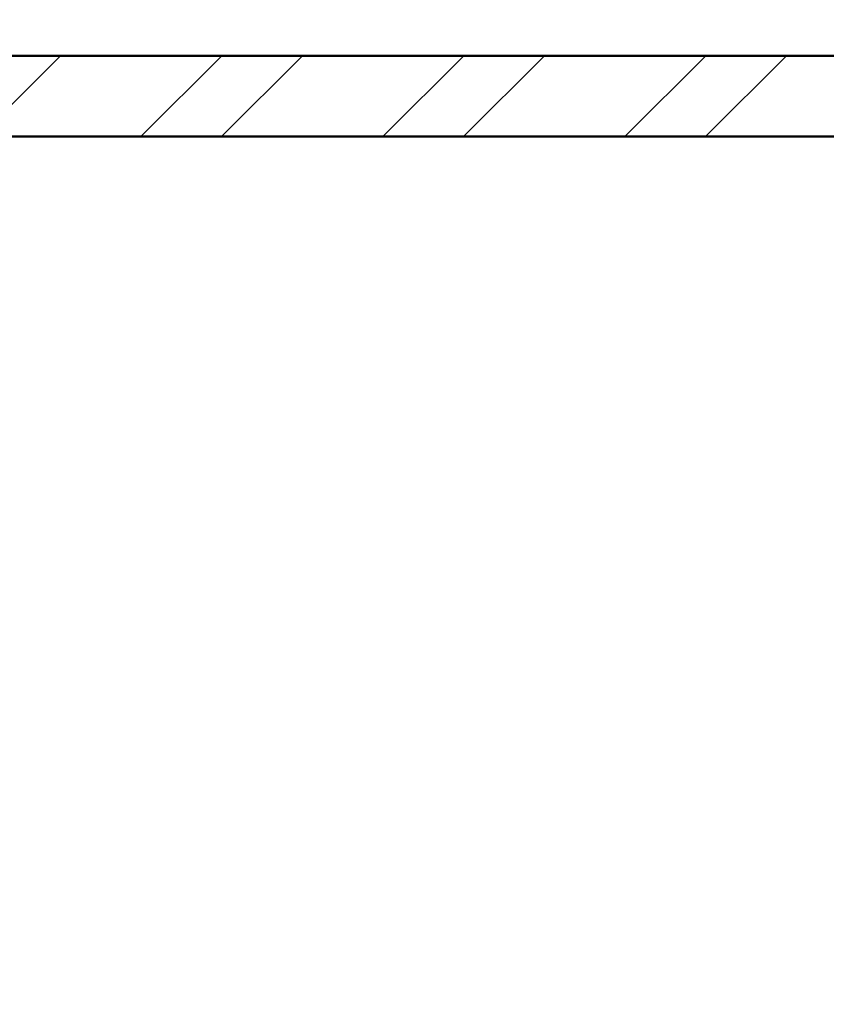
# Model space of a CAD drawing. Units: inches. Extents: x 1901 to 2863, y 888 to 2433.
# Tile 12 of 91: x 2199 to 2244, y 1403 to 1458. Entities that reach past the tile are written whole.
import ezdxf

# ---------------------------------------------------------------- set-up
doc = ezdxf.new("R2010")
doc.units = ezdxf.units.IN
doc.layers.add('A-WALL', color=7, linetype='Continuous', lineweight=50)
doc.layers.add('A-WALL-PATT', color=8, linetype='Continuous', lineweight=13)

msp = doc.modelspace()

# ---------------------------------------------------------------- hatches: boundary and pattern name
at = {"layer": 'A-WALL-PATT'}
h = msp.add_hatch(dxfattribs=at)
h.set_pattern_fill('ANSI32', color=256)
h.paths.add_polyline_path([(2192.501, 2274.134), (2141.264, 2274.134), (2141.264, 2269.634), (2192.501, 2269.634)])
h.paths.add_polyline_path([(2259.926, 2274.134), (2216.501, 2274.134), (2216.501, 2269.634), (2255.426, 2269.634), (2255.426, 2214.634), (2250.809, 2214.634), (2250.809, 2210.134), (2259.926, 2210.134), (2259.926, 2215.134), (2271.756, 2215.134), (2271.756, 2217.384), (2271.756, 2219.634), (2259.926, 2219.634)])
h.paths.add_polyline_path([(2171.426, 2269.634), (2166.926, 2269.634), (2166.926, 2219.634), (2121.238, 2219.634), (2121.238, 2215.134), (2166.926, 2215.134), (2166.926, 2083.134), (2161.807, 2083.134), (2161.807, 2078.634), (2171.426, 2078.634), (2176.996, 2078.634), (2176.996, 2080.884), (2176.996, 2083.134), (2171.426, 2083.134), (2171.426, 2210.134), (2230.912, 2210.134), (2230.912, 2212.384), (2230.912, 2214.634), (2171.426, 2214.634)])
h.paths.add_polyline_path([(2117.264, 2274.134), (2089.426, 2274.134), (2089.426, 2219.634), (2081.136, 2219.634), (2081.136, 2215.134), (2089.426, 2215.134), (2098.004, 2215.134), (2098.004, 2217.384), (2098.004, 2219.634), (2093.926, 2219.634), (2093.926, 2269.634), (2117.264, 2269.634), (2117.264, 2271.884)])
h.paths.add_polyline_path([(2343.426, 2219.634), (2329.295, 2219.634), (2329.295, 2215.134), (2338.926, 2215.134), (2338.926, 2184.739), (2343.426, 2184.739)])
h.paths.add_polyline_path([(2338.926, 2083.134), (2329.295, 2083.134), (2208.966, 2083.134), (2208.966, 2078.634), (2338.926, 2078.634)])
h.paths.add_polyline_path([(2343.426, 2136.739), (2338.926, 2136.739), (2338.926, 1872.634), (2343.426, 1872.634)])
h.paths.add_polyline_path([(2343.426, 1863.634), (2397.68, 1863.634), (2397.68, 1821.634), (2384.138, 1821.634), (2384.138, 1812.634), (2418.33, 1812.634), (2418.33, 1817.134), (2418.33, 1821.634), (2406.68, 1821.634), (2406.68, 1863.634), (2459.499, 1863.634), (2459.499, 1821.634), (2447.138, 1821.634), (2447.138, 1812.634), (2459.499, 1812.634), (2468.499, 1812.634), (2468.499, 1872.634), (2394.426, 1872.634), (2334.426, 1872.634), (2334.426, 1812.634), (2343.426, 1812.634), (2353.251, 1812.634), (2353.251, 1821.634), (2343.426, 1821.634)])
h.paths.add_polyline_path([(2510.014, 1872.634), (2468.499, 1872.634), (2468.499, 1868.134), (2510.014, 1868.134)])
h.paths.add_polyline_path([(2514.009, 1817.134), (2468.499, 1817.134), (2468.499, 1812.634), (2482.114, 1812.634), (2482.114, 1800.606), (2486.614, 1800.606), (2486.614, 1812.634), (2514.009, 1812.634)])
h.paths.add_polyline_path([(2299.247, 1814.884), (2299.247, 1817.134), (2295.926, 1817.134), (2295.926, 1854.169), (2293.676, 1854.169), (2291.426, 1854.169), (2291.426, 1817.134), (2266.109, 1817.134), (2266.109, 1812.634), (2299.247, 1812.634)])
h.paths.add_polyline_path([(2218.109, 1817.134), (2206.46, 1817.134), (2171.426, 1817.134), (2171.426, 1949.134), (2190.1, 1949.134), (2190.1, 1953.634), (2163.468, 1953.634), (2163.468, 1949.134), (2166.926, 1949.134), (2166.926, 1817.134), (2114.297, 1817.134), (2114.297, 1812.634), (2218.109, 1812.634)])
h.paths.add_polyline_path([(2029.426, 1970.922), (2024.926, 1970.922), (2024.926, 1912.717), (2029.426, 1912.717)])
h.paths.add_polyline_path([(2132.297, 1953.634), (2113.926, 1953.634), (2113.926, 1975.888), (2111.676, 1975.888), (2109.426, 1975.888), (2109.426, 1953.634), (2029.426, 1953.634), (2029.426, 1949.134), (2132.297, 1949.134)])
h.paths.add_polyline_path([(2029.426, 1853.606), (2029.31, 1853.606), (2029.31, 1853.606), (2029.426, 1853.606), (2029.426, 1864.717), (2024.926, 1864.717), (2024.926, 1812.634), (2066.297, 1812.634), (2066.297, 1814.884), (2066.297, 1817.134), (2029.426, 1817.134)])
h.paths.add_polyline_path([(2122.926, 2010.088), (2120.676, 2010.088), (2118.426, 2010.088), (2118.426, 2006.134), (2029.426, 2006.134), (2029.426, 2001.634), (2109.426, 2001.634), (2109.426, 1998.041), (2113.926, 1998.041), (2113.926, 2001.634), (2122.926, 2001.634)])
h.paths.add_polyline_path([(2029.426, 2031.376), (2024.926, 2031.376), (2024.926, 1994.922), (2027.176, 1994.922), (2029.426, 1994.922)])
h.paths.add_polyline_path([(2029.426, 2136.739), (2024.926, 2136.739), (2024.926, 2067.376), (2027.176, 2067.376), (2029.426, 2067.376)])
h.paths.add_polyline_path([(2125.618, 2083.134), (2029.426, 2083.134), (2029.426, 2078.634), (2118.426, 2078.634), (2118.426, 2030.715), (2122.926, 2030.715), (2122.926, 2078.634), (2125.618, 2078.634)])
h.paths.add_polyline_path([(2029.426, 2215.134), (2040.468, 2215.134), (2040.468, 2217.384), (2040.468, 2219.634), (2024.926, 2219.634), (2024.926, 2184.739), (2029.426, 2184.739), (2029.426, 2187.778)])
h.paths.add_polyline_path([(2686.426, 2274.134), (2659.284, 2274.134), (2659.284, 2269.634), (2681.926, 2269.634), (2681.926, 2219.634), (2676.816, 2219.634), (2676.816, 2215.134), (2681.926, 2215.134), (2697.011, 2215.134), (2697.011, 2217.384), (2697.011, 2219.634), (2686.426, 2219.634)])
h.paths.add_polyline_path([(2609.926, 2269.634), (2635.284, 2269.634), (2635.284, 2274.134), (2571.431, 2274.134), (2571.431, 2269.634), (2605.426, 2269.634), (2605.426, 2214.634), (2549.098, 2214.634), (2549.098, 2210.134), (2605.426, 2210.134), (2605.426, 2083.134), (2601.014, 2083.134), (2601.014, 2080.884), (2601.014, 2078.634), (2609.926, 2078.634), (2616.162, 2078.634), (2616.162, 2080.884), (2616.162, 2083.134), (2609.926, 2083.134), (2609.926, 2215.134), (2651.465, 2215.134), (2651.465, 2217.384), (2651.465, 2219.634), (2609.926, 2219.634)])
h.paths.add_polyline_path([(2521.426, 2269.634), (2547.431, 2269.634), (2547.431, 2271.884), (2547.431, 2274.134), (2516.926, 2274.134), (2516.926, 2219.634), (2506.41, 2219.634), (2506.41, 2215.134), (2516.926, 2215.134), (2516.926, 2210.134), (2525.402, 2210.134), (2525.402, 2212.384), (2525.402, 2214.634), (2521.426, 2214.634)])
h.paths.add_polyline_path([(2456.011, 2219.634), (2439.426, 2219.634), (2439.426, 2187.888), (2443.926, 2187.888), (2443.926, 2215.134), (2456.011, 2215.134)])
h.paths.add_polyline_path([(2752.926, 2219.634), (2739.485, 2219.634), (2739.485, 2215.134), (2748.426, 2215.134), (2748.426, 2187.888), (2752.926, 2187.888)])
h.paths.add_polyline_path([(2752.926, 2139.888), (2748.426, 2139.888), (2748.426, 2083.134), (2648.416, 2083.134), (2648.416, 2078.634), (2654.926, 2078.634), (2654.926, 2039.437), (2659.426, 2039.437), (2659.426, 2078.634), (2748.426, 2078.634), (2748.426, 2063.429), (2752.926, 2063.429)])
h.paths.add_polyline_path([(2752.926, 2010.634), (2659.426, 2010.634), (2659.426, 2015.652), (2654.926, 2015.652), (2654.926, 2010.634), (2605.426, 2010.634), (2605.426, 1920.967), (2609.926, 1920.967), (2609.926, 2006.134), (2748.426, 2006.134), (2748.426, 1982.466), (2752.926, 1982.466)])
h.paths.add_polyline_path([(2752.926, 2027.429), (2748.426, 2027.429), (2748.426, 2010.634), (2752.926, 2010.634)])
h.paths.add_polyline_path([(2748.426, 1886.134), (2609.926, 1886.134), (2609.926, 1889.719), (2605.426, 1889.719), (2605.426, 1861.262), (2609.926, 1861.262), (2609.926, 1881.634), (2748.426, 1881.634)])
h.paths.add_polyline_path([(2456.855, 2228.831), (2498.401, 2228.831), (2498.401, 2247.488), (2456.855, 2247.488)], flags=9)
h.paths.add_polyline_path([(2038.602, 2237.418), (2080.174, 2237.418), (2080.174, 2256.075), (2038.602, 2256.075)], flags=9)
h.paths.add_polyline_path([(2292.009, 1062.394), (2539.932, 1062.394), (2539.932, 1099.487), (2292.009, 1099.487)], flags=9)
h.paths.add_polyline_path([(2424.91, 1832.253), (2448.513, 1832.253), (2448.513, 1846.678), (2424.91, 1846.678)], flags=25)
h.paths.add_polyline_path([(2359.076, 1832.253), (2382.678, 1832.253), (2382.678, 1846.678), (2359.076, 1846.678)], flags=25)
h.paths.add_polyline_path([(2352.899, 1684.802), (2367.543, 1684.802), (2367.543, 1697.167), (2352.899, 1697.167)], flags=9)
h.paths.add_polyline_path([(2079.288, 1755.826), (2169.024, 1755.826), (2169.024, 1774.372), (2079.288, 1774.372)], flags=9)
h.paths.add_polyline_path([(2404.09, 1373.857), (2404.09, 1463.593), (2385.544, 1463.593), (2385.544, 1373.857)], flags=9)
h.paths.add_polyline_path([(2268.091, 2236.371), (2309.636, 2236.371), (2309.636, 2255.028), (2268.091, 2255.028)], flags=9)
h.paths.add_polyline_path([(2575.96, 1700.951), (2665.696, 1700.951), (2665.696, 1719.498), (2575.96, 1719.498)], flags=9)
h.paths.add_polyline_path([(2302.962, 1878.474), (2329.524, 1878.474), (2329.524, 1888.777), (2302.962, 1888.777)], flags=9)
h.paths.add_polyline_path([(2097.415, 2240.576), (2126.573, 2240.576), (2126.573, 2259.233), (2097.415, 2259.233)], flags=9)
h.paths.add_polyline_path([(2208.725, 2246.124), (2237.882, 2246.124), (2237.882, 2264.781), (2208.725, 2264.781)], flags=9)
h.paths.add_polyline_path([(2038.147, 1925.958), (2076.987, 1925.958), (2076.987, 1944.615), (2038.147, 1944.615)], flags=9)
h.paths.add_polyline_path([(2239.144, 1926.672), (2288.465, 1926.672), (2288.465, 1945.329), (2239.144, 1945.329)], flags=9)
h.paths.add_polyline_path([(2175.429, 2007.33), (2212.356, 2007.33), (2212.356, 2025.987), (2175.429, 2025.987)], flags=9)
h.paths.add_polyline_path([(2225.034, 2091.794), (2263.875, 2091.794), (2263.875, 2110.451), (2225.034, 2110.451)], flags=9)
h.paths.add_polyline_path([(2035.398, 2098.478), (2074.238, 2098.478), (2074.238, 2117.135), (2035.398, 2117.135)], flags=9)
h.paths.add_polyline_path([(2050.102, 2029.209), (2083.26, 2029.209), (2083.26, 2047.866), (2050.102, 2047.866)], flags=9)
h.paths.add_polyline_path([(2069.677, 1956.719), (2098.835, 1956.719), (2098.835, 1975.376), (2069.677, 1975.376)], flags=25)
h.paths.add_polyline_path([(2328.62, 1753.336), (2361.663, 1753.336), (2361.663, 1771.993), (2328.62, 1771.993)], flags=9)
h.paths.add_polyline_path([(2395.162, 2060.888), (2395.162, 2140.654), (2378.676, 2140.654), (2378.676, 2060.888)], flags=9)
h.paths.add_polyline_path([(2463.728, 2059.02), (2492.886, 2059.02), (2492.886, 2077.677), (2463.728, 2077.677)], flags=9)
h.paths.add_polyline_path([(2458.027, 2181.536), (2496.868, 2181.536), (2496.868, 2200.194), (2458.027, 2200.194)], flags=9)
h.paths.add_polyline_path([(2527.577, 2243.074), (2556.735, 2243.074), (2556.735, 2261.731), (2527.577, 2261.731)], flags=9)
h.paths.add_polyline_path([(2694.461, 2232.767), (2736.033, 2232.767), (2736.033, 2251.425), (2694.461, 2251.425)], flags=9)
h.paths.add_polyline_path([(2637.821, 2249.225), (2666.979, 2249.225), (2666.979, 2267.882), (2637.821, 2267.882)], flags=9)
h.paths.add_polyline_path([(2623.687, 2183.541), (2662.528, 2183.541), (2662.528, 2202.199), (2623.687, 2202.199)], flags=9)
h.paths.add_polyline_path([(2691.965, 2021.5), (2725.124, 2021.5), (2725.124, 2040.157), (2691.965, 2040.157)], flags=9)
h.paths.add_polyline_path([(2621.043, 1975.912), (2662.335, 1975.912), (2662.335, 1994.569), (2621.043, 1994.569)], flags=25)
h.paths.add_polyline_path([(2479.032, 1927.62), (2519.844, 1927.62), (2519.844, 1946.277), (2479.032, 1946.277)], flags=9)
h.paths.add_polyline_path([(2670.941, 1849.076), (2716.005, 1849.076), (2716.005, 1867.734), (2670.941, 1867.734)], flags=9)
h.paths.add_polyline_path([(2523.613, 1782.956), (2550.175, 1782.956), (2550.175, 1793.26), (2523.613, 1793.26)], flags=9)
h.paths.add_polyline_path([(2450.841, 1207.331), (2492.386, 1207.331), (2492.386, 1225.989), (2450.841, 1225.989)], flags=9)
h.paths.add_polyline_path([(2527.751, 1203.841), (2556.908, 1203.841), (2556.908, 1222.499), (2527.751, 1222.499)], flags=9)
h.paths.add_polyline_path([(2639.111, 1207.2), (2668.268, 1207.2), (2668.268, 1225.857), (2639.111, 1225.857)], flags=9)
h.paths.add_polyline_path([(2692.594, 1218.965), (2734.167, 1218.965), (2734.167, 1237.623), (2692.594, 1237.623)], flags=9)
h.paths.add_polyline_path([(2669.266, 1366.329), (2708.106, 1366.329), (2708.106, 1384.987), (2669.266, 1384.987)], flags=9)
h.paths.add_polyline_path([(2463.313, 1358.031), (2502.153, 1358.031), (2502.153, 1376.688), (2463.313, 1376.688)], flags=9)
h.paths.add_polyline_path([(2494.725, 1449.963), (2531.652, 1449.963), (2531.652, 1468.62), (2494.725, 1468.62)], flags=9)
h.paths.add_polyline_path([(2675.565, 1422.157), (2708.724, 1422.157), (2708.724, 1440.815), (2675.565, 1440.815)], flags=9)
h.paths.add_polyline_path([(2685.634, 1493.891), (2714.792, 1493.891), (2714.792, 1512.548), (2685.634, 1512.548)], flags=9)
h.paths.add_polyline_path([(2686.805, 1529.913), (2725.645, 1529.913), (2725.645, 1548.57), (2686.805, 1548.57)], flags=9)
h.paths.add_polyline_path([(2503.651, 1537.991), (2552.972, 1537.991), (2552.972, 1556.648), (2503.651, 1556.648)], flags=9)
h.paths.add_polyline_path([(2291.713, 1643.504), (2318.275, 1643.504), (2318.275, 1653.807), (2291.713, 1653.807)], flags=9)
h.paths.add_polyline_path([(2450.626, 1610.52), (2477.189, 1610.52), (2477.189, 1620.824), (2450.626, 1620.824)], flags=9)
h.paths.add_polyline_path([(2359.985, 1551.814), (2422.253, 1551.814), (2422.253, 1562.117), (2359.985, 1562.117)], flags=9)
h.paths.add_polyline_path([(2280.106, 1249.006), (2321.651, 1249.006), (2321.651, 1267.663), (2280.106, 1267.663)], flags=9)
h.paths.add_polyline_path([(2164.057, 1274.232), (2193.215, 1274.232), (2193.215, 1292.889), (2164.057, 1292.889)], flags=9)
h.paths.add_polyline_path([(2118.21, 1277.694), (2151.252, 1277.694), (2151.252, 1296.351), (2118.21, 1296.351)], flags=9)
h.paths.add_polyline_path([(2031.946, 1268.529), (2073.519, 1268.529), (2073.519, 1287.187), (2031.946, 1287.187)], flags=9)
h.paths.add_polyline_path([(2050.199, 1409.079), (2089.04, 1409.079), (2089.04, 1427.736), (2050.199, 1427.736)], flags=9)
h.paths.add_polyline_path([(2243.743, 1421.032), (2282.584, 1421.032), (2282.584, 1439.689), (2243.743, 1439.689)], flags=9)
h.paths.add_polyline_path([(2190.746, 1509.769), (2231.558, 1509.769), (2231.558, 1528.426), (2190.746, 1528.426)], flags=9)
h.paths.add_polyline_path([(2058.392, 1475.415), (2091.55, 1475.415), (2091.55, 1494.073), (2058.392, 1494.073)], flags=9)
h.paths.add_polyline_path([(2062.447, 1553.09), (2091.605, 1553.09), (2091.605, 1571.747), (2062.447, 1571.747)], flags=9)
h.paths.add_polyline_path([(2219.524, 1590.365), (2266.147, 1590.365), (2266.147, 1609.022), (2219.524, 1609.022)], flags=9)
h.paths.add_polyline_path([(2041.072, 1584.188), (2079.912, 1584.188), (2079.912, 1602.845), (2041.072, 1602.845)], flags=9)
h = msp.add_hatch(dxfattribs=at)
h.set_pattern_fill('ANSI32', color=256)
h.paths.add_polyline_path([(2443.926, 2139.888), (2439.426, 2139.888), (2439.426, 2069.348), (2441.676, 2069.348), (2443.926, 2069.348), (2443.926, 2078.634), (2521.926, 2078.634), (2521.926, 2075.067), (2524.176, 2075.067), (2526.426, 2075.067), (2526.426, 2078.634), (2571.755, 2078.634), (2571.755, 2080.884), (2571.755, 2083.134), (2443.926, 2083.134)])
h.paths.add_polyline_path([(2526.426, 2054.634), (2524.176, 2054.634), (2521.926, 2054.634), (2521.926, 2030.634), (2443.926, 2030.634), (2443.926, 2045.348), (2439.426, 2045.348), (2439.426, 1983.867), (2443.926, 1983.867), (2443.926, 2026.134), (2521.926, 2026.134), (2526.426, 2026.134)])
h.paths.add_polyline_path([(2443.926, 1923.867), (2439.426, 1923.867), (2439.426, 1872.634), (2443.926, 1872.634)])
h.paths.add_polyline_path([(2636.233, 1766.134), (2609.926, 1766.134), (2609.926, 1779.785), (2605.426, 1779.785), (2605.426, 1766.134), (2486.614, 1766.134), (2486.614, 1770.671), (2482.114, 1770.671), (2482.114, 1766.134), (2482.114, 1761.634), (2636.233, 1761.634), (2636.233, 1763.884)])
h.paths.add_polyline_path([(2519.536, 1663.384), (2519.536, 1665.634), (2494.926, 1665.634), (2481.831, 1665.634), (2481.831, 1663.384), (2481.831, 1661.134), (2490.426, 1661.134), (2490.426, 1640.157), (2494.926, 1640.157), (2494.926, 1661.134), (2519.536, 1661.134)])
h.paths.add_polyline_path([(2443.926, 1712.134), (2443.926, 1716.634), (2414.464, 1716.634), (2414.464, 1712.134), (2439.426, 1712.134), (2439.426, 1545.507), (2443.926, 1545.507), (2443.926, 1661.134), (2448.475, 1661.134), (2448.475, 1665.634), (2443.926, 1665.634)])
h.paths.add_polyline_path([(2343.426, 1712.134), (2365.525, 1712.134), (2365.525, 1714.384), (2365.525, 1716.634), (2333.871, 1716.634), (2333.871, 1714.384), (2333.871, 1712.134), (2338.926, 1712.134), (2338.926, 1575.634), (2338.926, 1545.507), (2343.426, 1545.507), (2343.426, 1547.507), (2343.426, 1580.134)])
h.paths.add_polyline_path([(2752.926, 1665.634), (2579.536, 1665.634), (2579.536, 1661.134), (2615.926, 1661.134), (2615.926, 1529.134), (2598.931, 1529.134), (2598.931, 1524.634), (2623.127, 1524.634), (2623.127, 1526.884), (2623.127, 1529.134), (2620.426, 1529.134), (2620.426, 1661.134), (2748.426, 1661.134), (2748.426, 1633.499), (2752.926, 1633.499)])
h.paths.add_polyline_path([(2752.926, 1419.929), (2748.426, 1419.929), (2748.426, 1400.134), (2659.426, 1400.134), (2659.426, 1444.333), (2657.176, 1444.333), (2654.926, 1444.333), (2654.926, 1400.134), (2643.649, 1400.134), (2643.649, 1395.634), (2748.426, 1395.634), (2748.426, 1364.035), (2752.926, 1364.035)])
h.paths.add_polyline_path([(2752.926, 1492.878), (2748.426, 1492.878), (2748.426, 1476.634), (2667.426, 1476.634), (2667.426, 1479.71), (2665.176, 1479.71), (2662.926, 1479.71), (2662.926, 1476.634), (2654.926, 1476.634), (2654.926, 1469.536), (2659.426, 1469.536), (2659.426, 1472.134), (2748.426, 1472.134), (2748.426, 1455.929), (2752.926, 1455.929)])
h.paths.add_polyline_path([(2752.926, 1304.035), (2748.426, 1304.035), (2748.426, 1263.634), (2738.66, 1263.634), (2738.66, 1259.134), (2752.926, 1259.134)])
h.paths.add_polyline_path([(2685.926, 1259.134), (2695.49, 1259.134), (2695.49, 1261.384), (2695.49, 1263.634), (2677.837, 1263.634), (2677.837, 1261.384), (2677.837, 1259.134), (2681.426, 1259.134), (2681.426, 1203.634), (2653.277, 1203.634), (2653.277, 1199.134), (2685.926, 1199.134), (2685.926, 1203.634)])
h.paths.add_polyline_path([(2609.426, 1395.634), (2611.848, 1395.634), (2611.848, 1400.134), (2598.888, 1400.134), (2598.888, 1397.884), (2598.888, 1395.634), (2604.926, 1395.634), (2604.926, 1268.134), (2554.726, 1268.134), (2554.726, 1265.884), (2554.726, 1263.634), (2604.926, 1263.634), (2604.926, 1203.634), (2571.306, 1203.634), (2571.306, 1199.134), (2604.926, 1199.134), (2629.277, 1199.134), (2629.277, 1201.384), (2629.277, 1203.634), (2609.426, 1203.634), (2609.426, 1258.634), (2609.426, 1259.134), (2654.804, 1259.134), (2654.804, 1263.634), (2609.426, 1263.634)])
h.paths.add_polyline_path([(2443.926, 1304.035), (2439.426, 1304.035), (2439.426, 1259.134), (2443.926, 1259.134), (2456.16, 1259.134), (2456.16, 1261.384), (2456.16, 1263.634), (2443.926, 1263.634)])
h.paths.add_polyline_path([(2525.426, 1263.634), (2531.778, 1263.634), (2531.778, 1268.134), (2520.926, 1268.134), (2520.926, 1263.634), (2511.409, 1263.634), (2511.409, 1259.134), (2520.926, 1259.134), (2520.926, 1199.134), (2547.306, 1199.134), (2547.306, 1201.384), (2547.306, 1203.634), (2525.426, 1203.634)])
h.paths.add_polyline_path([(2443.926, 1434.842), (2439.426, 1434.842), (2439.426, 1364.035), (2441.676, 1364.035), (2443.926, 1364.035)])
h.paths.add_polyline_path([(2567.134, 1400.134), (2443.926, 1400.134), (2443.926, 1395.634), (2567.134, 1395.634)])
h.paths.add_polyline_path([(2443.926, 1545.507), (2439.426, 1545.507), (2439.426, 1494.842), (2443.926, 1494.842)])
h.paths.add_polyline_path([(2494.926, 1553.349), (2492.676, 1553.349), (2490.426, 1553.349), (2490.426, 1524.634), (2494.926, 1524.634), (2525.936, 1524.634), (2525.936, 1526.884), (2525.936, 1529.134), (2494.926, 1529.134)])
h.paths.add_polyline_path([(2752.926, 1573.499), (2748.426, 1573.499), (2748.426, 1529.134), (2657.759, 1529.134), (2657.759, 1524.634), (2662.926, 1524.634), (2662.926, 1498.631), (2667.426, 1498.631), (2667.426, 1524.634), (2748.426, 1524.634), (2748.426, 1516.878), (2752.926, 1516.878)])
h.paths.add_polyline_path([(2038.602, 2237.418), (2080.174, 2237.418), (2080.174, 2256.075), (2038.602, 2256.075)], flags=9)
h.paths.add_polyline_path([(2292.009, 1062.394), (2539.932, 1062.394), (2539.932, 1099.487), (2292.009, 1099.487)], flags=9)
h.paths.add_polyline_path([(2424.91, 1832.253), (2448.513, 1832.253), (2448.513, 1846.678), (2424.91, 1846.678)], flags=9)
h.paths.add_polyline_path([(2359.076, 1832.253), (2382.678, 1832.253), (2382.678, 1846.678), (2359.076, 1846.678)], flags=9)
h.paths.add_polyline_path([(2352.899, 1684.802), (2367.543, 1684.802), (2367.543, 1697.167), (2352.899, 1697.167)], flags=9)
h.paths.add_polyline_path([(2079.288, 1755.826), (2169.024, 1755.826), (2169.024, 1774.372), (2079.288, 1774.372)], flags=9)
h.paths.add_polyline_path([(2404.09, 1373.857), (2404.09, 1463.593), (2385.544, 1463.593), (2385.544, 1373.857)], flags=9)
h.paths.add_polyline_path([(2268.091, 2236.371), (2309.636, 2236.371), (2309.636, 2255.028), (2268.091, 2255.028)], flags=9)
h.paths.add_polyline_path([(2575.96, 1700.951), (2665.696, 1700.951), (2665.696, 1719.498), (2575.96, 1719.498)], flags=9)
h.paths.add_polyline_path([(2302.962, 1878.474), (2329.524, 1878.474), (2329.524, 1888.777), (2302.962, 1888.777)], flags=9)
h.paths.add_polyline_path([(2097.415, 2240.576), (2126.573, 2240.576), (2126.573, 2259.233), (2097.415, 2259.233)], flags=9)
h.paths.add_polyline_path([(2208.725, 2246.124), (2237.882, 2246.124), (2237.882, 2264.781), (2208.725, 2264.781)], flags=9)
h.paths.add_polyline_path([(2038.147, 1925.958), (2076.987, 1925.958), (2076.987, 1944.615), (2038.147, 1944.615)], flags=9)
h.paths.add_polyline_path([(2239.144, 1926.672), (2288.465, 1926.672), (2288.465, 1945.329), (2239.144, 1945.329)], flags=9)
h.paths.add_polyline_path([(2175.429, 2007.33), (2212.356, 2007.33), (2212.356, 2025.987), (2175.429, 2025.987)], flags=9)
h.paths.add_polyline_path([(2225.034, 2091.794), (2263.875, 2091.794), (2263.875, 2110.451), (2225.034, 2110.451)], flags=9)
h.paths.add_polyline_path([(2035.398, 2098.478), (2074.238, 2098.478), (2074.238, 2117.135), (2035.398, 2117.135)], flags=9)
h.paths.add_polyline_path([(2050.102, 2029.209), (2083.26, 2029.209), (2083.26, 2047.866), (2050.102, 2047.866)], flags=9)
h.paths.add_polyline_path([(2069.677, 1956.719), (2098.835, 1956.719), (2098.835, 1975.376), (2069.677, 1975.376)], flags=9)
h.paths.add_polyline_path([(2328.62, 1753.336), (2361.663, 1753.336), (2361.663, 1771.993), (2328.62, 1771.993)], flags=9)
h.paths.add_polyline_path([(2395.162, 2060.888), (2395.162, 2140.654), (2378.676, 2140.654), (2378.676, 2060.888)], flags=9)
h.paths.add_polyline_path([(2463.728, 2059.02), (2492.886, 2059.02), (2492.886, 2077.677), (2463.728, 2077.677)], flags=9)
h.paths.add_polyline_path([(2458.027, 2181.536), (2496.868, 2181.536), (2496.868, 2200.194), (2458.027, 2200.194)], flags=9)
h.paths.add_polyline_path([(2456.855, 2228.831), (2498.401, 2228.831), (2498.401, 2247.488), (2456.855, 2247.488)], flags=9)
h.paths.add_polyline_path([(2527.577, 2243.074), (2556.735, 2243.074), (2556.735, 2261.731), (2527.577, 2261.731)], flags=9)
h.paths.add_polyline_path([(2694.461, 2232.767), (2736.033, 2232.767), (2736.033, 2251.425), (2694.461, 2251.425)], flags=9)
h.paths.add_polyline_path([(2637.821, 2249.225), (2666.979, 2249.225), (2666.979, 2267.882), (2637.821, 2267.882)], flags=9)
h.paths.add_polyline_path([(2623.687, 2183.541), (2662.528, 2183.541), (2662.528, 2202.199), (2623.687, 2202.199)], flags=9)
h.paths.add_polyline_path([(2691.965, 2021.5), (2725.124, 2021.5), (2725.124, 2040.157), (2691.965, 2040.157)], flags=9)
h.paths.add_polyline_path([(2621.043, 1975.912), (2662.335, 1975.912), (2662.335, 1994.569), (2621.043, 1994.569)], flags=9)
h.paths.add_polyline_path([(2479.032, 1927.62), (2519.844, 1927.62), (2519.844, 1946.277), (2479.032, 1946.277)], flags=9)
h.paths.add_polyline_path([(2670.941, 1849.076), (2716.005, 1849.076), (2716.005, 1867.734), (2670.941, 1867.734)], flags=9)
h.paths.add_polyline_path([(2523.613, 1782.956), (2550.175, 1782.956), (2550.175, 1793.26), (2523.613, 1793.26)], flags=9)
h.paths.add_polyline_path([(2450.841, 1207.331), (2492.386, 1207.331), (2492.386, 1225.989), (2450.841, 1225.989)], flags=9)
h.paths.add_polyline_path([(2527.751, 1203.841), (2556.908, 1203.841), (2556.908, 1222.499), (2527.751, 1222.499)], flags=9)
h.paths.add_polyline_path([(2639.111, 1207.2), (2668.268, 1207.2), (2668.268, 1225.857), (2639.111, 1225.857)], flags=9)
h.paths.add_polyline_path([(2692.594, 1218.965), (2734.167, 1218.965), (2734.167, 1237.623), (2692.594, 1237.623)], flags=9)
h.paths.add_polyline_path([(2669.266, 1366.329), (2708.106, 1366.329), (2708.106, 1384.987), (2669.266, 1384.987)], flags=25)
h.paths.add_polyline_path([(2463.313, 1358.031), (2502.153, 1358.031), (2502.153, 1376.688), (2463.313, 1376.688)], flags=9)
h.paths.add_polyline_path([(2494.725, 1449.963), (2531.652, 1449.963), (2531.652, 1468.62), (2494.725, 1468.62)], flags=9)
h.paths.add_polyline_path([(2675.565, 1422.157), (2708.724, 1422.157), (2708.724, 1440.815), (2675.565, 1440.815)], flags=25)
h.paths.add_polyline_path([(2685.634, 1493.891), (2714.792, 1493.891), (2714.792, 1512.548), (2685.634, 1512.548)], flags=9)
h.paths.add_polyline_path([(2686.805, 1529.913), (2725.645, 1529.913), (2725.645, 1548.57), (2686.805, 1548.57)], flags=25)
h.paths.add_polyline_path([(2503.651, 1537.991), (2552.972, 1537.991), (2552.972, 1556.648), (2503.651, 1556.648)], flags=9)
h.paths.add_polyline_path([(2291.713, 1643.504), (2318.275, 1643.504), (2318.275, 1653.807), (2291.713, 1653.807)], flags=9)
h.paths.add_polyline_path([(2450.626, 1610.52), (2477.189, 1610.52), (2477.189, 1620.824), (2450.626, 1620.824)], flags=9)
h.paths.add_polyline_path([(2359.985, 1551.814), (2422.253, 1551.814), (2422.253, 1562.117), (2359.985, 1562.117)], flags=9)
h.paths.add_polyline_path([(2280.106, 1249.006), (2321.651, 1249.006), (2321.651, 1267.663), (2280.106, 1267.663)], flags=9)
h.paths.add_polyline_path([(2164.057, 1274.232), (2193.215, 1274.232), (2193.215, 1292.889), (2164.057, 1292.889)], flags=9)
h.paths.add_polyline_path([(2118.21, 1277.694), (2151.252, 1277.694), (2151.252, 1296.351), (2118.21, 1296.351)], flags=9)
h.paths.add_polyline_path([(2031.946, 1268.529), (2073.519, 1268.529), (2073.519, 1287.187), (2031.946, 1287.187)], flags=9)
h.paths.add_polyline_path([(2050.199, 1409.079), (2089.04, 1409.079), (2089.04, 1427.736), (2050.199, 1427.736)], flags=9)
h.paths.add_polyline_path([(2243.743, 1421.032), (2282.584, 1421.032), (2282.584, 1439.689), (2243.743, 1439.689)], flags=9)
h.paths.add_polyline_path([(2190.746, 1509.769), (2231.558, 1509.769), (2231.558, 1528.426), (2190.746, 1528.426)], flags=9)
h.paths.add_polyline_path([(2058.392, 1475.415), (2091.55, 1475.415), (2091.55, 1494.073), (2058.392, 1494.073)], flags=9)
h.paths.add_polyline_path([(2062.447, 1553.09), (2091.605, 1553.09), (2091.605, 1571.747), (2062.447, 1571.747)], flags=9)
h.paths.add_polyline_path([(2219.524, 1590.365), (2266.147, 1590.365), (2266.147, 1609.022), (2219.524, 1609.022)], flags=9)
h.paths.add_polyline_path([(2041.072, 1584.188), (2079.912, 1584.188), (2079.912, 1602.845), (2041.072, 1602.845)], flags=9)
h = msp.add_hatch(dxfattribs=at)
h.set_pattern_fill('ANSI32', color=256)
h.paths.add_polyline_path([(2182.933, 1716.634), (2024.926, 1716.634), (2024.926, 1681.702), (2029.326, 1681.702), (2029.326, 1712.134), (2154.326, 1712.134), (2154.326, 1580.134), (2148.524, 1580.134), (2148.524, 1577.884), (2148.524, 1575.634), (2194.93, 1575.634), (2194.93, 1580.134), (2158.826, 1580.134), (2158.826, 1712.134), (2182.933, 1712.134)])
h.paths.add_polyline_path([(2301.069, 1716.634), (2242.933, 1716.634), (2242.933, 1712.134), (2283.826, 1712.134), (2283.826, 1685.535), (2288.326, 1685.535), (2288.326, 1712.134), (2301.069, 1712.134)])
h.paths.add_polyline_path([(2288.326, 1600.411), (2286.076, 1600.411), (2283.826, 1600.411), (2283.826, 1580.134), (2270.601, 1580.134), (2270.601, 1575.634), (2288.326, 1575.634)])
h.paths.add_polyline_path([(2295.926, 1953.634), (2271.447, 1953.634), (2271.447, 1949.134), (2291.426, 1949.134), (2291.426, 1941.244), (2295.926, 1941.244)])
h.paths.add_polyline_path([(2098.376, 1244.134), (2082.326, 1244.134), (2082.326, 1302.134), (2086.523, 1302.134), (2086.523, 1306.634), (2067.456, 1306.634), (2067.456, 1302.134), (2077.826, 1302.134), (2077.826, 1239.634), (2098.376, 1239.634), (2098.376, 1241.884)])
h.paths.add_polyline_path([(2217.308, 1306.634), (2158.826, 1306.634), (2158.826, 1451.634), (2162.716, 1451.634), (2162.716, 1453.884), (2162.716, 1456.134), (2154.326, 1456.134), (2154.326, 1443.134), (2151.91, 1443.134), (2151.91, 1438.634), (2154.326, 1438.634), (2154.326, 1306.634), (2109.307, 1306.634), (2109.307, 1304.384), (2109.307, 1302.134), (2154.326, 1302.134), (2154.326, 1244.134), (2122.376, 1244.134), (2122.376, 1239.634), (2154.326, 1239.634), (2154.326, 1223.634), (2163.326, 1223.634), (2181.008, 1223.634), (2181.008, 1225.884), (2181.008, 1228.134), (2163.326, 1228.134), (2163.326, 1258.222), (2158.826, 1258.222), (2158.826, 1302.134), (2217.308, 1302.134)])
h.paths.add_polyline_path([(2259.991, 1306.634), (2238.299, 1306.634), (2238.299, 1304.384), (2238.299, 1302.134), (2242.826, 1302.134), (2242.826, 1228.134), (2205.008, 1228.134), (2205.008, 1223.634), (2247.326, 1223.634), (2247.326, 1302.134), (2259.991, 1302.134), (2259.991, 1304.384)])
h.paths.add_polyline_path([(2343.426, 1361.697), (2338.926, 1361.697), (2338.926, 1306.634), (2322.38, 1306.634), (2322.38, 1302.134), (2343.426, 1302.134)])
h.paths.add_polyline_path([(2343.426, 1470.397), (2338.926, 1470.397), (2338.926, 1456.134), (2193.726, 1456.134), (2193.726, 1453.884), (2193.726, 1451.634), (2338.926, 1451.634), (2338.926, 1421.697), (2343.426, 1421.697)])
h.paths.add_polyline_path([(2343.426, 1545.507), (2338.926, 1545.507), (2338.926, 1530.397), (2343.426, 1530.397)])
h.paths.add_polyline_path([(2029.326, 1466.83), (2024.926, 1466.83), (2024.926, 1409.825), (2029.326, 1409.825)])
h.paths.add_polyline_path([(2122.843, 1440.884), (2122.843, 1443.134), (2121.826, 1443.134), (2121.826, 1498.183), (2119.576, 1498.183), (2117.326, 1498.183), (2117.326, 1443.134), (2029.326, 1443.134), (2029.326, 1438.634), (2122.843, 1438.634)])
h.paths.add_polyline_path([(2029.326, 1543.053), (2024.926, 1543.053), (2024.926, 1502.83), (2029.326, 1502.83)])
h.paths.add_polyline_path([(2029.326, 1621.702), (2024.926, 1621.702), (2024.926, 1567.053), (2027.126, 1567.053), (2029.326, 1567.053), (2029.326, 1575.634), (2109.326, 1575.634), (2109.326, 1554.715), (2113.826, 1554.715), (2113.826, 1575.634), (2115.805, 1575.634), (2115.805, 1577.884), (2115.805, 1580.134), (2029.326, 1580.134)])
h.paths.add_polyline_path([(2121.826, 1527.634), (2117.326, 1527.634), (2113.826, 1527.634), (2113.826, 1533.011), (2111.576, 1533.011), (2109.326, 1533.011), (2109.326, 1527.634), (2029.326, 1527.634), (2029.326, 1523.134), (2117.326, 1523.134), (2117.326, 1519.43), (2121.826, 1519.43)])
h.paths.add_polyline_path([(2029.326, 1349.825), (2024.926, 1349.825), (2024.926, 1302.134), (2036.277, 1302.134), (2036.277, 1306.634), (2029.326, 1306.634)])

# ---------------------------------------------------------------- linework, layer by layer
at = {"layer": 'A-WALL'}
for p, q in [((2338.926, 1456.134), (2193.726, 1456.134)), ((2338.926, 1451.634), (2192.282, 1451.634))]:
    msp.add_line(p, q, dxfattribs=at)

doc.saveas('drawing.dxf')
